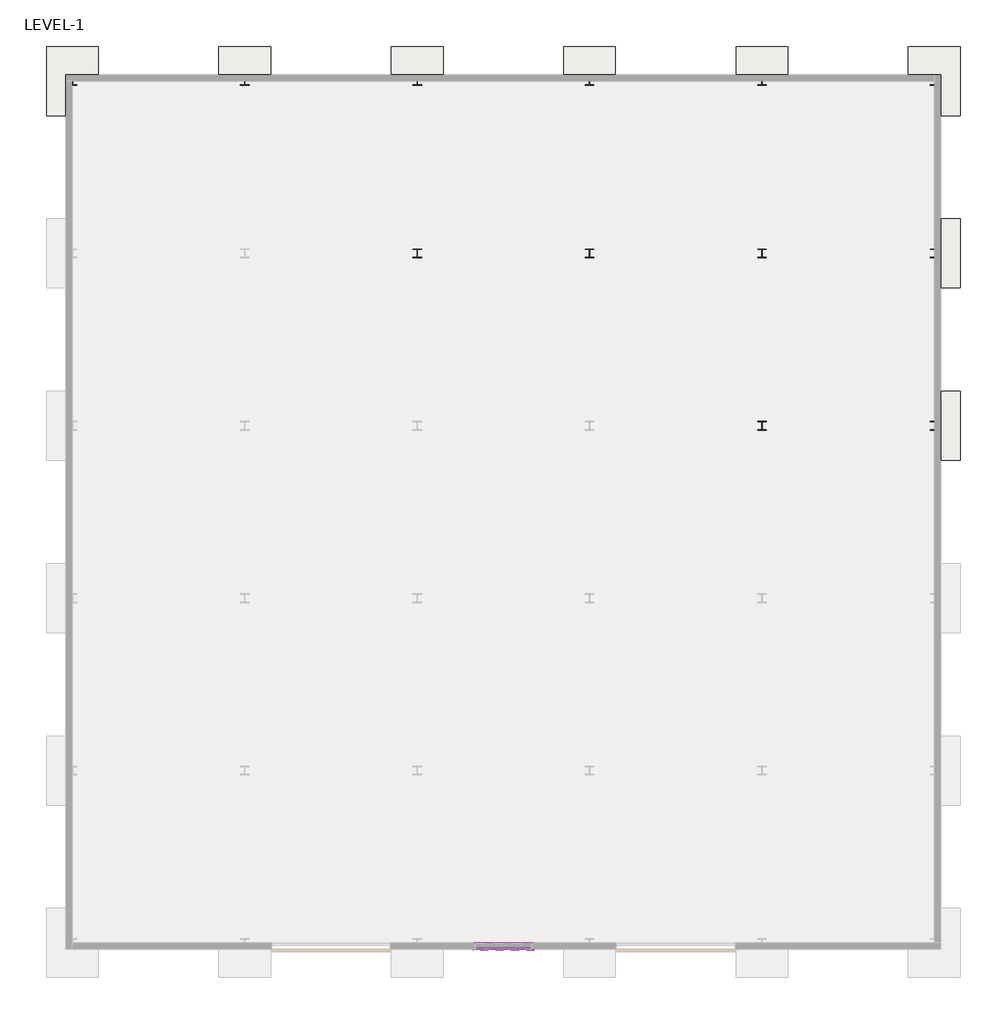
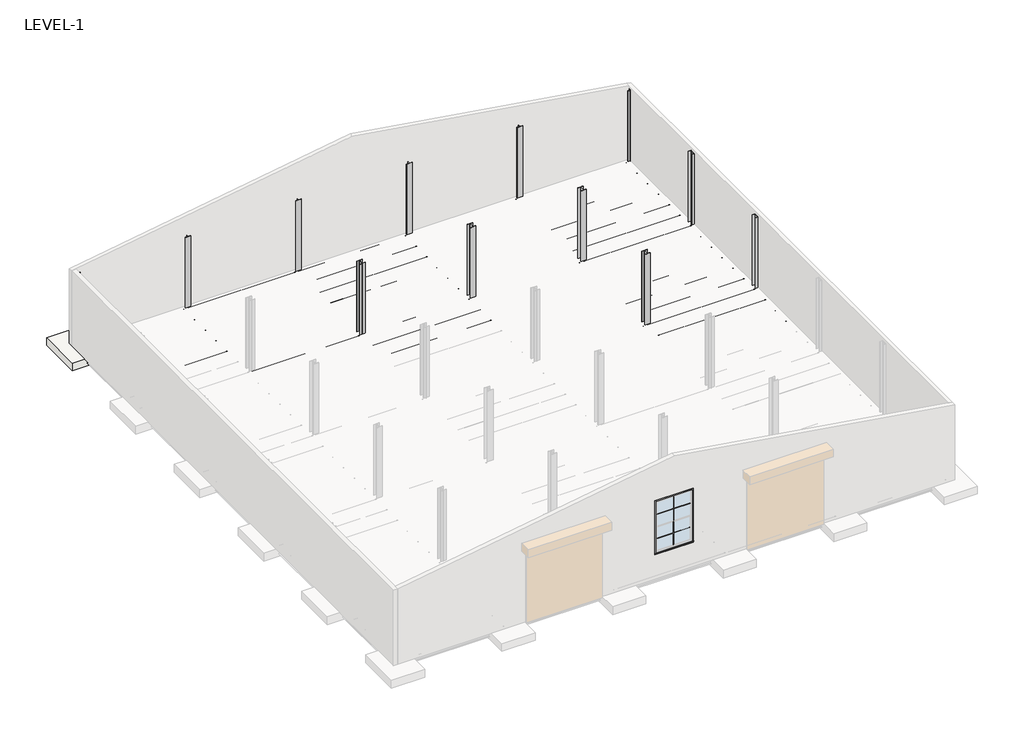
# One storey, part 3 of 3: 64 beams, 12 columns, 12 slabs, 4 proxies.
"""IFC4 building model written with IfcOpenShell, lengths in millimetres."""

from ifc_helpers import new_model, si_unit, origin, place, context, project, spatial, transform, mapped, element, save
from components import ub_universal_beams_ub305x165x40_15f88fa9, ub_universal_beams_ub305x165x40_f918ae41, ub_universal_beams_ub305x165x40_f15b2736, ub_universal_beams_ub305x165x40_44492b97, m_muntin_pattern_2x2_m_muntin_pattern_2x2_665a5da2, m_trim_window_exterior_flat_with_sill_5e8edc4f, m_trim_window_interior_flat_picture_frame_e5a503a4, uc_universal_columns_column_uc305x305x97_11a20181, slab_7b69f09a

model = new_model("IFC4")

# Units and contexts
model_context = context("Model", 3, world=origin())
ifc_project = project(units=[si_unit("LENGTHUNIT", "METRE", prefix="MILLI")], contexts=[model_context])

# Site, building, storey
site = spatial("IfcSite", under=ifc_project)
building = spatial("IfcBuilding", under=site)
storey = spatial("IfcBuildingStorey", under=building, Name="LEVEL-1", Elevation=0.0)

# Beams
placement = place(None, origin())
ub_universal_beams_ub305x165x40_shape = ub_universal_beams_ub305x165x40_15f88fa9(model_context)
element("IfcBeam", 1, ObjectType="UB-Universal Beams : UB305x165x40", at=placement, inside=storey, context=model_context, shape_type="MappedRepresentation", body=[
    mapped(ub_universal_beams_ub305x165x40_shape, transform((-15492.3332854, 15135.5234105, -151.7), x_axis=(1.0, 0.0, 0.0), y_axis=(0.0, 1.0, 0.0), z_axis=(0.0, 0.0, 1.0))),
])
element("IfcBeam", 2, ObjectType="UB-Universal Beams : UB305x165x40", at=placement, inside=storey, context=model_context, shape_type="MappedRepresentation", body=[
    mapped(ub_universal_beams_ub305x165x40_shape, transform((-15492.3332854, 14119.5234105, -151.7), x_axis=(1.0, 0.0, 0.0), y_axis=(0.0, 1.0, 0.0), z_axis=(0.0, 0.0, 1.0))),
])
element("IfcBeam", 3, ObjectType="UB-Universal Beams : UB305x165x40", at=placement, inside=storey, context=model_context, shape_type="MappedRepresentation", body=[
    mapped(ub_universal_beams_ub305x165x40_shape, transform((-15492.3332854, 13103.5234105, -151.7), x_axis=(1.0, 0.0, 0.0), y_axis=(0.0, 1.0, 0.0), z_axis=(0.0, 0.0, 1.0))),
])
element("IfcBeam", 4, ObjectType="UB-Universal Beams : UB305x165x40", at=placement, inside=storey, context=model_context, shape_type="MappedRepresentation", body=[
    mapped(ub_universal_beams_ub305x165x40_shape, transform((-15492.3332854, 12087.5234105, -151.7), x_axis=(1.0, 0.0, 0.0), y_axis=(0.0, 1.0, 0.0), z_axis=(0.0, 0.0, 1.0))),
])
element("IfcBeam", 5, ObjectType="UB-Universal Beams : UB305x165x40", at=placement, inside=storey, context=model_context, shape_type="MappedRepresentation", body=[
    mapped(ub_universal_beams_ub305x165x40_shape, transform((-3300.3332854, 15135.5234105, -151.7), x_axis=(1.0, 0.0, 0.0), y_axis=(0.0, 1.0, 0.0), z_axis=(0.0, 0.0, 1.0))),
])
element("IfcBeam", 6, ObjectType="UB-Universal Beams : UB305x165x40", at=placement, inside=storey, context=model_context, shape_type="MappedRepresentation", body=[
    mapped(ub_universal_beams_ub305x165x40_shape, transform((-3300.3332854, 14119.5234105, -151.7), x_axis=(1.0, 0.0, 0.0), y_axis=(0.0, 1.0, 0.0), z_axis=(0.0, 0.0, 1.0))),
])
element("IfcBeam", 7, ObjectType="UB-Universal Beams : UB305x165x40", at=placement, inside=storey, context=model_context, shape_type="MappedRepresentation", body=[
    mapped(ub_universal_beams_ub305x165x40_shape, transform((-3300.3332854, 13103.5234105, -151.7), x_axis=(1.0, 0.0, 0.0), y_axis=(0.0, 1.0, 0.0), z_axis=(0.0, 0.0, 1.0))),
])
element("IfcBeam", 8, ObjectType="UB-Universal Beams : UB305x165x40", at=placement, inside=storey, context=model_context, shape_type="MappedRepresentation", body=[
    mapped(ub_universal_beams_ub305x165x40_shape, transform((-3300.3332854, 12087.5234105, -151.7), x_axis=(1.0, 0.0, 0.0), y_axis=(0.0, 1.0, 0.0), z_axis=(0.0, 0.0, 1.0))),
])
element("IfcBeam", 9, ObjectType="UB-Universal Beams : UB305x165x40", at=placement, inside=storey, context=model_context, shape_type="MappedRepresentation", body=[
    mapped(ub_universal_beams_ub305x165x40_shape, transform((-3300.3332854, 11071.5234105, -151.7), x_axis=(1.0, 0.0, 0.0), y_axis=(0.0, 1.0, 0.0), z_axis=(0.0, 0.0, 1.0))),
])
element("IfcBeam", 10, ObjectType="UB-Universal Beams : UB305x165x40", at=placement, inside=storey, context=model_context, shape_type="MappedRepresentation", body=[
    mapped(ub_universal_beams_ub305x165x40_shape, transform((-3300.3332854, 9039.5234105, -151.7), x_axis=(1.0, 0.0, 0.0), y_axis=(0.0, 1.0, 0.0), z_axis=(0.0, 0.0, 1.0))),
])
element("IfcBeam", 11, ObjectType="UB-Universal Beams : UB305x165x40", at=placement, inside=storey, context=model_context, shape_type="MappedRepresentation", body=[
    mapped(ub_universal_beams_ub305x165x40_shape, transform((-3300.3332854, 8023.5234105, -151.7), x_axis=(1.0, 0.0, 0.0), y_axis=(0.0, 1.0, 0.0), z_axis=(0.0, 0.0, 1.0))),
])
element("IfcBeam", 12, ObjectType="UB-Universal Beams : UB305x165x40", at=placement, inside=storey, context=model_context, shape_type="MappedRepresentation", body=[
    mapped(ub_universal_beams_ub305x165x40_shape, transform((8891.6667146, 15135.5234105, -151.7), x_axis=(1.0, 0.0, 0.0), y_axis=(0.0, 1.0, 0.0), z_axis=(0.0, 0.0, 1.0))),
])
element("IfcBeam", 13, ObjectType="UB-Universal Beams : UB305x165x40", at=placement, inside=storey, context=model_context, shape_type="MappedRepresentation", body=[
    mapped(ub_universal_beams_ub305x165x40_shape, transform((8891.6667146, 14119.5234105, -151.7), x_axis=(1.0, 0.0, 0.0), y_axis=(0.0, 1.0, 0.0), z_axis=(0.0, 0.0, 1.0))),
])
element("IfcBeam", 14, ObjectType="UB-Universal Beams : UB305x165x40", at=placement, inside=storey, context=model_context, shape_type="MappedRepresentation", body=[
    mapped(ub_universal_beams_ub305x165x40_shape, transform((8891.6667146, 13103.5234105, -151.7), x_axis=(1.0, 0.0, 0.0), y_axis=(0.0, 1.0, 0.0), z_axis=(0.0, 0.0, 1.0))),
])
element("IfcBeam", 15, ObjectType="UB-Universal Beams : UB305x165x40", at=placement, inside=storey, context=model_context, shape_type="MappedRepresentation", body=[
    mapped(ub_universal_beams_ub305x165x40_shape, transform((8891.6667146, 12087.5234105, -151.7), x_axis=(1.0, 0.0, 0.0), y_axis=(0.0, 1.0, 0.0), z_axis=(0.0, 0.0, 1.0))),
])
element("IfcBeam", 16, ObjectType="UB-Universal Beams : UB305x165x40", at=placement, inside=storey, context=model_context, shape_type="MappedRepresentation", body=[
    mapped(ub_universal_beams_ub305x165x40_shape, transform((8891.6667146, 11071.5234105, -151.7), x_axis=(1.0, 0.0, 0.0), y_axis=(0.0, 1.0, 0.0), z_axis=(0.0, 0.0, 1.0))),
])
element("IfcBeam", 17, ObjectType="UB-Universal Beams : UB305x165x40", at=placement, inside=storey, context=model_context, shape_type="MappedRepresentation", body=[
    mapped(ub_universal_beams_ub305x165x40_shape, transform((8891.6667146, 9039.5234105, -151.7), x_axis=(1.0, 0.0, 0.0), y_axis=(0.0, 1.0, 0.0), z_axis=(0.0, 0.0, 1.0))),
])
element("IfcBeam", 18, ObjectType="UB-Universal Beams : UB305x165x40", at=placement, inside=storey, context=model_context, shape_type="MappedRepresentation", body=[
    mapped(ub_universal_beams_ub305x165x40_shape, transform((8891.6667146, 8023.5234105, -151.7), x_axis=(1.0, 0.0, 0.0), y_axis=(0.0, 1.0, 0.0), z_axis=(0.0, 0.0, 1.0))),
])
element("IfcBeam", 19, ObjectType="UB-Universal Beams : UB305x165x40", at=placement, inside=storey, context=model_context, shape_type="MappedRepresentation", body=[
    mapped(ub_universal_beams_ub305x165x40_shape, transform((8891.6667146, 7007.5234105, -151.7), x_axis=(1.0, 0.0, 0.0), y_axis=(0.0, 1.0, 0.0), z_axis=(0.0, 0.0, 1.0))),
])
element("IfcBeam", 20, ObjectType="UB-Universal Beams : UB305x165x40", at=placement, inside=storey, context=model_context, shape_type="MappedRepresentation", body=[
    mapped(ub_universal_beams_ub305x165x40_shape, transform((8891.6667146, 5991.5234105, -151.7), x_axis=(1.0, 0.0, 0.0), y_axis=(0.0, 1.0, 0.0), z_axis=(0.0, 0.0, 1.0))),
])
element("IfcBeam", 21, ObjectType="UB-Universal Beams : UB305x165x40", at=placement, inside=storey, context=model_context, shape_type="MappedRepresentation", body=[
    mapped(ub_universal_beams_ub305x165x40_shape, transform((8891.6667146, 4975.5234105, -151.7), x_axis=(1.0, 0.0, 0.0), y_axis=(0.0, 1.0, 0.0), z_axis=(0.0, 0.0, 1.0))),
])
element("IfcBeam", 22, ObjectType="UB-Universal Beams : UB305x165x40", at=placement, inside=storey, context=model_context, shape_type="MappedRepresentation", body=[
    mapped(ub_universal_beams_ub305x165x40_shape, transform((8891.6667146, 2943.5234105, -151.7), x_axis=(1.0, 0.0, 0.0), y_axis=(0.0, 1.0, 0.0), z_axis=(0.0, 0.0, 1.0))),
])
element("IfcBeam", 23, ObjectType="UB-Universal Beams : UB305x165x40", at=placement, inside=storey, context=model_context, shape_type="MappedRepresentation", body=[
    mapped(ub_universal_beams_ub305x165x40_shape, transform((8891.6667146, 1927.5234105, -151.7), x_axis=(1.0, 0.0, 0.0), y_axis=(0.0, 1.0, 0.0), z_axis=(0.0, 0.0, 1.0))),
])
element("IfcBeam", 24, ObjectType="UB-Universal Beams : UB305x165x40", at=placement, inside=storey, context=model_context, shape_type="MappedRepresentation", body=[
    mapped(ub_universal_beams_ub305x165x40_shape, transform((8891.6667146, 911.5234105, -151.7), x_axis=(1.0, 0.0, 0.0), y_axis=(0.0, 1.0, 0.0), z_axis=(0.0, 0.0, 1.0))),
])
element("IfcBeam", 25, ObjectType="UB-Universal Beams : UB305x165x40", at=placement, inside=storey, context=model_context, shape_type="MappedRepresentation", body=[
    mapped(ub_universal_beams_ub305x165x40_shape, transform((-7364.3332854, 13103.5234105, -151.7), x_axis=(0.0, -1.0, 0.0), y_axis=(1.0, 0.0, 0.0), z_axis=(0.0, 0.0, 1.0))),
])
element("IfcBeam", 26, ObjectType="UB-Universal Beams : UB305x165x40", at=placement, inside=storey, context=model_context, shape_type="MappedRepresentation", body=[
    mapped(ub_universal_beams_ub305x165x40_shape, transform((-8380.3332854, 13103.5234105, -151.7), x_axis=(0.0, -1.0, 0.0), y_axis=(1.0, 0.0, 0.0), z_axis=(0.0, 0.0, 1.0))),
])
element("IfcBeam", 27, ObjectType="UB-Universal Beams : UB305x165x40", at=placement, inside=storey, context=model_context, shape_type="MappedRepresentation", body=[
    mapped(ub_universal_beams_ub305x165x40_shape, transform((-9396.3332854, 13103.5234105, -151.7), x_axis=(0.0, -1.0, 0.0), y_axis=(1.0, 0.0, 0.0), z_axis=(0.0, 0.0, 1.0))),
])
element("IfcBeam", 28, ObjectType="UB-Universal Beams : UB305x165x40", at=placement, inside=storey, context=model_context, shape_type="MappedRepresentation", body=[
    mapped(ub_universal_beams_ub305x165x40_shape, transform((-10412.3332854, 13103.5234105, -151.7), x_axis=(0.0, -1.0, 0.0), y_axis=(1.0, 0.0, 0.0), z_axis=(0.0, 0.0, 1.0))),
])
element("IfcBeam", 29, ObjectType="UB-Universal Beams : UB305x165x40", at=placement, inside=storey, context=model_context, shape_type="MappedRepresentation", body=[
    mapped(ub_universal_beams_ub305x165x40_shape, transform((-11428.3332854, 13103.5234105, -151.7), x_axis=(0.0, -1.0, 0.0), y_axis=(1.0, 0.0, 0.0), z_axis=(0.0, 0.0, 1.0))),
])
element("IfcBeam", 30, ObjectType="UB-Universal Beams : UB305x165x40", at=placement, inside=storey, context=model_context, shape_type="MappedRepresentation", body=[
    mapped(ub_universal_beams_ub305x165x40_shape, transform((4827.6667146, 13103.5234105, -151.7), x_axis=(0.0, -1.0, 0.0), y_axis=(1.0, 0.0, 0.0), z_axis=(0.0, 0.0, 1.0))),
])
element("IfcBeam", 31, ObjectType="UB-Universal Beams : UB305x165x40", at=placement, inside=storey, context=model_context, shape_type="MappedRepresentation", body=[
    mapped(ub_universal_beams_ub305x165x40_shape, transform((3811.6667146, 13103.5234105, -151.7), x_axis=(0.0, -1.0, 0.0), y_axis=(1.0, 0.0, 0.0), z_axis=(0.0, 0.0, 1.0))),
])
element("IfcBeam", 32, ObjectType="UB-Universal Beams : UB305x165x40", at=placement, inside=storey, context=model_context, shape_type="MappedRepresentation", body=[
    mapped(ub_universal_beams_ub305x165x40_shape, transform((2795.6667146, 13103.5234105, -151.7), x_axis=(0.0, -1.0, 0.0), y_axis=(1.0, 0.0, 0.0), z_axis=(0.0, 0.0, 1.0))),
])
element("IfcBeam", 33, ObjectType="UB-Universal Beams : UB305x165x40", at=placement, inside=storey, context=model_context, shape_type="MappedRepresentation", body=[
    mapped(ub_universal_beams_ub305x165x40_shape, transform((1779.6667146, 13103.5234105, -151.7), x_axis=(0.0, -1.0, 0.0), y_axis=(1.0, 0.0, 0.0), z_axis=(0.0, 0.0, 1.0))),
])
element("IfcBeam", 34, ObjectType="UB-Universal Beams : UB305x165x40", at=placement, inside=storey, context=model_context, shape_type="MappedRepresentation", body=[
    mapped(ub_universal_beams_ub305x165x40_shape, transform((763.6667146, 13103.5234105, -151.7), x_axis=(0.0, -1.0, 0.0), y_axis=(1.0, 0.0, 0.0), z_axis=(0.0, 0.0, 1.0))),
])
element("IfcBeam", 35, ObjectType="UB-Universal Beams : UB305x165x40", at=placement, inside=storey, context=model_context, shape_type="MappedRepresentation", body=[
    mapped(ub_universal_beams_ub305x165x40_shape, transform((4827.6667146, 7007.5234105, -151.7), x_axis=(0.0, -1.0, 0.0), y_axis=(1.0, 0.0, 0.0), z_axis=(0.0, 0.0, 1.0))),
])
element("IfcBeam", 36, ObjectType="UB-Universal Beams : UB305x165x40", at=placement, inside=storey, context=model_context, shape_type="MappedRepresentation", body=[
    mapped(ub_universal_beams_ub305x165x40_shape, transform((3811.6667146, 7007.5234105, -151.7), x_axis=(0.0, -1.0, 0.0), y_axis=(1.0, 0.0, 0.0), z_axis=(0.0, 0.0, 1.0))),
])
element("IfcBeam", 37, ObjectType="UB-Universal Beams : UB305x165x40", at=placement, inside=storey, context=model_context, shape_type="MappedRepresentation", body=[
    mapped(ub_universal_beams_ub305x165x40_shape, transform((2795.6667146, 7007.5234105, -151.7), x_axis=(0.0, -1.0, 0.0), y_axis=(1.0, 0.0, 0.0), z_axis=(0.0, 0.0, 1.0))),
])
element("IfcBeam", 38, ObjectType="UB-Universal Beams : UB305x165x40", at=placement, inside=storey, context=model_context, shape_type="MappedRepresentation", body=[
    mapped(ub_universal_beams_ub305x165x40_shape, transform((1779.6667146, 7007.5234105, -151.7), x_axis=(0.0, -1.0, 0.0), y_axis=(1.0, 0.0, 0.0), z_axis=(0.0, 0.0, 1.0))),
])
element("IfcBeam", 39, ObjectType="UB-Universal Beams : UB305x165x40", at=placement, inside=storey, context=model_context, shape_type="MappedRepresentation", body=[
    mapped(ub_universal_beams_ub305x165x40_shape, transform((763.6667146, 7007.5234105, -151.7), x_axis=(0.0, -1.0, 0.0), y_axis=(1.0, 0.0, 0.0), z_axis=(0.0, 0.0, 1.0))),
])
element("IfcBeam", 40, ObjectType="UB-Universal Beams : UB305x165x40", at=placement, inside=storey, context=model_context, shape_type="MappedRepresentation", body=[
    mapped(ub_universal_beams_ub305x165x40_shape, transform((4827.6667146, 911.5234105, -151.7), x_axis=(0.0, -1.0, 0.0), y_axis=(1.0, 0.0, 0.0), z_axis=(0.0, 0.0, 1.0))),
])
element("IfcBeam", 41, ObjectType="UB-Universal Beams : UB305x165x40", at=placement, inside=storey, context=model_context, shape_type="MappedRepresentation", body=[
    mapped(ub_universal_beams_ub305x165x40_shape, transform((3811.6667146, 911.5234105, -151.7), x_axis=(0.0, -1.0, 0.0), y_axis=(1.0, 0.0, 0.0), z_axis=(0.0, 0.0, 1.0))),
])
element("IfcBeam", 42, ObjectType="UB-Universal Beams : UB305x165x40", at=placement, inside=storey, context=model_context, shape_type="MappedRepresentation", body=[
    mapped(ub_universal_beams_ub305x165x40_shape, transform((2795.6667146, 911.5234105, -151.7), x_axis=(0.0, -1.0, 0.0), y_axis=(1.0, 0.0, 0.0), z_axis=(0.0, 0.0, 1.0))),
])
element("IfcBeam", 43, ObjectType="UB-Universal Beams : UB305x165x40", at=placement, inside=storey, context=model_context, shape_type="MappedRepresentation", body=[
    mapped(ub_universal_beams_ub305x165x40_shape, transform((1779.6667146, 911.5234105, -151.7), x_axis=(0.0, -1.0, 0.0), y_axis=(1.0, 0.0, 0.0), z_axis=(0.0, 0.0, 1.0))),
])
element("IfcBeam", 44, ObjectType="UB-Universal Beams : UB305x165x40", at=placement, inside=storey, context=model_context, shape_type="MappedRepresentation", body=[
    mapped(ub_universal_beams_ub305x165x40_shape, transform((763.6667146, 911.5234105, -151.7), x_axis=(0.0, -1.0, 0.0), y_axis=(1.0, 0.0, 0.0), z_axis=(0.0, 0.0, 1.0))),
])
element("IfcBeam", 45, ObjectType="UB-Universal Beams : UB305x165x40", at=placement, inside=storey, context=model_context, shape_type="MappedRepresentation", body=[
    mapped(ub_universal_beams_ub305x165x40_shape, transform((2795.6667146, 3959.5234105, -151.7), x_axis=(1.0, 0.0, 0.0), y_axis=(0.0, 1.0, 0.0), z_axis=(0.0, 0.0, 1.0))),
])
element("IfcBeam", 46, ObjectType="UB-Universal Beams : UB305x165x40", at=placement, inside=storey, context=model_context, shape_type="MappedRepresentation", body=[
    mapped(ub_universal_beams_ub305x165x40_shape, transform((8891.6667146, 3959.5234105, -151.7), x_axis=(1.0, 0.0, 0.0), y_axis=(0.0, 1.0, 0.0), z_axis=(0.0, 0.0, 1.0))),
])
element("IfcBeam", 47, ObjectType="UB-Universal Beams : UB305x165x40", at=placement, inside=storey, context=model_context, shape_type="MappedRepresentation", body=[
    mapped(ub_universal_beams_ub305x165x40_shape, transform((-9396.3332854, 10055.5234105, -151.7), x_axis=(1.0, 0.0, 0.0), y_axis=(0.0, 1.0, 0.0), z_axis=(0.0, 0.0, 1.0))),
])
element("IfcBeam", 48, ObjectType="UB-Universal Beams : UB305x165x40", at=placement, inside=storey, context=model_context, shape_type="MappedRepresentation", body=[
    mapped(ub_universal_beams_ub305x165x40_shape, transform((-3300.3332854, 10055.5234105, -151.7), x_axis=(1.0, 0.0, 0.0), y_axis=(0.0, 1.0, 0.0), z_axis=(0.0, 0.0, 1.0))),
])
element("IfcBeam", 49, ObjectType="UB-Universal Beams : UB305x165x40", at=placement, inside=storey, context=model_context, shape_type="MappedRepresentation", body=[
    mapped(ub_universal_beams_ub305x165x40_shape, transform((2795.6667146, 10055.5234105, -151.7), x_axis=(1.0, 0.0, 0.0), y_axis=(0.0, 1.0, 0.0), z_axis=(0.0, 0.0, 1.0))),
])
element("IfcBeam", 50, ObjectType="UB-Universal Beams : UB305x165x40", at=placement, inside=storey, context=model_context, shape_type="MappedRepresentation", body=[
    mapped(ub_universal_beams_ub305x165x40_shape, transform((8891.6667146, 10055.5234105, -151.7), x_axis=(1.0, 0.0, 0.0), y_axis=(0.0, 1.0, 0.0), z_axis=(0.0, 0.0, 1.0))),
])
element("IfcBeam", 51, ObjectType="UB-Universal Beams : UB305x165x40", at=placement, inside=storey, context=model_context, shape_type="MappedRepresentation", body=[
    mapped(ub_universal_beams_ub305x165x40_shape, transform((-9396.3332854, 16151.5234105, -151.7), x_axis=(1.0, 0.0, 0.0), y_axis=(0.0, 1.0, 0.0), z_axis=(0.0, 0.0, 1.0))),
])
element("IfcBeam", 52, ObjectType="UB-Universal Beams : UB305x165x40", at=placement, inside=storey, context=model_context, shape_type="MappedRepresentation", body=[
    mapped(ub_universal_beams_ub305x165x40_shape, transform((-3300.3332854, 16151.5234105, -151.7), x_axis=(1.0, 0.0, 0.0), y_axis=(0.0, 1.0, 0.0), z_axis=(0.0, 0.0, 1.0))),
])
element("IfcBeam", 53, ObjectType="UB-Universal Beams : UB305x165x40", at=placement, inside=storey, context=model_context, shape_type="MappedRepresentation", body=[
    mapped(ub_universal_beams_ub305x165x40_shape, transform((2795.6667146, 16151.5234105, -151.7), x_axis=(1.0, 0.0, 0.0), y_axis=(0.0, 1.0, 0.0), z_axis=(0.0, 0.0, 1.0))),
])
element("IfcBeam", 54, ObjectType="UB-Universal Beams : UB305x165x40", at=placement, inside=storey, context=model_context, shape_type="MappedRepresentation", body=[
    mapped(ub_universal_beams_ub305x165x40_shape, transform((8891.6667146, 16151.5234105, -151.7), x_axis=(1.0, 0.0, 0.0), y_axis=(0.0, 1.0, 0.0), z_axis=(0.0, 0.0, 1.0))),
])
ub_universal_beams_ub305x165x40_2_shape = ub_universal_beams_ub305x165x40_f918ae41(model_context)
element("IfcBeam", 55, ObjectType="UB-Universal Beams : UB305x165x40", at=placement, inside=storey, context=model_context, shape_type="MappedRepresentation", body=[
    mapped(ub_universal_beams_ub305x165x40_2_shape, transform((11939.6667146, 911.5234105, -151.7), x_axis=(0.0, 1.0, 0.0), y_axis=(-1.0, 0.0, 0.0), z_axis=(0.0, 0.0, 1.0))),
])
element("IfcBeam", 56, ObjectType="UB-Universal Beams : UB305x165x40", at=placement, inside=storey, context=model_context, shape_type="MappedRepresentation", body=[
    mapped(ub_universal_beams_ub305x165x40_2_shape, transform((11939.6667146, 7007.5234105, -151.7), x_axis=(0.0, 1.0, 0.0), y_axis=(-1.0, 0.0, 0.0), z_axis=(0.0, 0.0, 1.0))),
])
element("IfcBeam", 57, ObjectType="UB-Universal Beams : UB305x165x40", at=placement, inside=storey, context=model_context, shape_type="MappedRepresentation", body=[
    mapped(ub_universal_beams_ub305x165x40_2_shape, transform((5843.6667146, 911.5234105, -151.7), x_axis=(0.0, 1.0, 0.0), y_axis=(-1.0, 0.0, 0.0), z_axis=(0.0, 0.0, 1.0))),
])
element("IfcBeam", 58, ObjectType="UB-Universal Beams : UB305x165x40", at=placement, inside=storey, context=model_context, shape_type="MappedRepresentation", body=[
    mapped(ub_universal_beams_ub305x165x40_2_shape, transform((5843.6667146, 7007.5234105, -151.7), x_axis=(0.0, 1.0, 0.0), y_axis=(-1.0, 0.0, 0.0), z_axis=(0.0, 0.0, 1.0))),
])
ub_universal_beams_ub305x165x40_3_shape = ub_universal_beams_ub305x165x40_f15b2736(model_context)
element("IfcBeam", 59, ObjectType="UB-Universal Beams : UB305x165x40", at=placement, inside=storey, context=model_context, shape_type="MappedRepresentation", body=[
    mapped(ub_universal_beams_ub305x165x40_3_shape, transform((-15549.3308854, 16151.5234105, -151.7), x_axis=(1.0, 0.0, 0.0), y_axis=(0.0, 1.0, 0.0), z_axis=(0.0, 0.0, 1.0))),
])
ub_universal_beams_ub305x165x40_4_shape = ub_universal_beams_ub305x165x40_44492b97(model_context)
element("IfcBeam", 60, ObjectType="UB-Universal Beams : UB305x165x40", at=placement, inside=storey, context=model_context, shape_type="MappedRepresentation", body=[
    mapped(ub_universal_beams_ub305x165x40_4_shape, transform((11939.6667146, 13160.6734105, -151.7), x_axis=(0.0, 1.0, 0.0), y_axis=(-1.0, 0.0, 0.0), z_axis=(0.0, 0.0, 1.0))),
])
element("IfcBeam", 61, ObjectType="UB-Universal Beams : UB305x165x40", at=placement, inside=storey, context=model_context, shape_type="MappedRepresentation", body=[
    mapped(ub_universal_beams_ub305x165x40_4_shape, transform((5843.6667146, 13160.6734105, -151.7), x_axis=(0.0, 1.0, 0.0), y_axis=(-1.0, 0.0, 0.0), z_axis=(0.0, 0.0, 1.0))),
])
element("IfcBeam", 62, ObjectType="UB-Universal Beams : UB305x165x40", at=placement, inside=storey, context=model_context, shape_type="MappedRepresentation", body=[
    mapped(ub_universal_beams_ub305x165x40_4_shape, transform((-252.3332854, 13160.6734105, -151.7), x_axis=(0.0, 1.0, 0.0), y_axis=(-1.0, 0.0, 0.0), z_axis=(0.0, 0.0, 1.0))),
])
element("IfcBeam", 63, ObjectType="UB-Universal Beams : UB305x165x40", at=placement, inside=storey, context=model_context, shape_type="MappedRepresentation", body=[
    mapped(ub_universal_beams_ub305x165x40_4_shape, transform((-6348.3332854, 13160.6734105, -151.7), x_axis=(0.0, 1.0, 0.0), y_axis=(-1.0, 0.0, 0.0), z_axis=(0.0, 0.0, 1.0))),
])
element("IfcBeam", 64, ObjectType="UB-Universal Beams : UB305x165x40", at=placement, inside=storey, context=model_context, shape_type="MappedRepresentation", body=[
    mapped(ub_universal_beams_ub305x165x40_4_shape, transform((-12444.3332854, 13160.6734105, -151.7), x_axis=(0.0, 1.0, 0.0), y_axis=(-1.0, 0.0, 0.0), z_axis=(0.0, 0.0, 1.0))),
])

# Proxies
m_muntin_pattern_2x2_m_muntin_pattern_2x2_shape = m_muntin_pattern_2x2_m_muntin_pattern_2x2_665a5da2(model_context)
element("IfcBuildingElementProxy", 65, Name="M_Muntin Pattern_2x2 : M_Muntin Pattern_2x2", ObjectType="M_Muntin Pattern_2x2 : M_Muntin Pattern_2x2", at=placement, inside=storey, context=model_context, shape_type="MappedRepresentation", body=[
    mapped(m_muntin_pattern_2x2_m_muntin_pattern_2x2_shape, transform((-3300.3332854, -14522.1515895, 3035.1090152), x_axis=(-1.0, 0.0, 0.0), y_axis=(0.0, -1.0, 0.0), z_axis=(0.0, 0.0, 1.0))),
])
element("IfcBuildingElementProxy", 66, Name="M_Muntin Pattern_2x2 : M_Muntin Pattern_2x2", ObjectType="M_Muntin Pattern_2x2 : M_Muntin Pattern_2x2", at=placement, inside=storey, context=model_context, shape_type="MappedRepresentation", body=[
    mapped(m_muntin_pattern_2x2_m_muntin_pattern_2x2_shape, transform((-3300.3332854, -14477.7015895, 1589.0840152), x_axis=(-1.0, 0.0, 0.0), y_axis=(0.0, -1.0, 0.0), z_axis=(0.0, 0.0, 1.0))),
])
m_trim_window_exterior_flat_with_sill_shape = m_trim_window_exterior_flat_with_sill_5e8edc4f(model_context)
element("IfcBuildingElementProxy", 67, Name="M_Trim-Window-Exterior-Flat : with Sill", ObjectType="M_Trim-Window-Exterior-Flat : with Sill", at=placement, inside=storey, context=model_context, shape_type="MappedRepresentation", body=[
    mapped(m_trim_window_exterior_flat_with_sill_shape, transform((-3300.3332854, -14557.0765895, 4512.8840152), x_axis=(1.0, 0.0, 0.0), y_axis=(0.0, 0.0, 1.0), z_axis=(0.0, -1.0, 0.0))),
])
m_trim_window_interior_flat_picture_frame_shape = m_trim_window_interior_flat_picture_frame_e5a503a4(model_context)
element("IfcBuildingElementProxy", 68, Name="M_Trim-Window-Interior-Flat : Picture Frame", ObjectType="M_Trim-Window-Interior-Flat : Picture Frame", at=placement, inside=storey, context=model_context, shape_type="MappedRepresentation", body=[
    mapped(m_trim_window_interior_flat_picture_frame_shape, transform((-3300.3332854, -14328.4765895, 4512.8840152), x_axis=(-1.0, 0.0, 0.0), y_axis=(0.0, 0.0, 1.0), z_axis=(0.0, 1.0, 0.0))),
])

# Columns
uc_universal_columns_column_uc305x305x97_shape = uc_universal_columns_column_uc305x305x97_11a20181(model_context)
element("IfcColumn", 69, ObjectType="UC-Universal Columns-Column : UC305x305x97", at=placement, inside=storey, context=model_context, shape_type="MappedRepresentation", body=[
    mapped(uc_universal_columns_column_uc305x305x97_shape, transform((11939.6667146, 3959.5234105, 0.0), x_axis=(1.0, 0.0, 0.0), y_axis=(0.0, 1.0, 0.0), z_axis=(0.0, 0.0, 1.0))),
])
element("IfcColumn", 70, ObjectType="UC-Universal Columns-Column : UC305x305x97", at=placement, inside=storey, context=model_context, shape_type="MappedRepresentation", body=[
    mapped(uc_universal_columns_column_uc305x305x97_shape, transform((5843.6667146, 3959.5234105, 0.0), x_axis=(1.0, 0.0, 0.0), y_axis=(0.0, 1.0, 0.0), z_axis=(0.0, 0.0, 1.0))),
])
element("IfcColumn", 71, ObjectType="UC-Universal Columns-Column : UC305x305x97", at=placement, inside=storey, context=model_context, shape_type="MappedRepresentation", body=[
    mapped(uc_universal_columns_column_uc305x305x97_shape, transform((11939.6667146, 10055.5234105, 0.0), x_axis=(1.0, 0.0, 0.0), y_axis=(0.0, 1.0, 0.0), z_axis=(0.0, 0.0, 1.0))),
])
element("IfcColumn", 72, ObjectType="UC-Universal Columns-Column : UC305x305x97", at=placement, inside=storey, context=model_context, shape_type="MappedRepresentation", body=[
    mapped(uc_universal_columns_column_uc305x305x97_shape, transform((5843.6667146, 10055.5234105, 0.0), x_axis=(1.0, 0.0, 0.0), y_axis=(0.0, 1.0, 0.0), z_axis=(0.0, 0.0, 1.0))),
])
element("IfcColumn", 73, ObjectType="UC-Universal Columns-Column : UC305x305x97", at=placement, inside=storey, context=model_context, shape_type="MappedRepresentation", body=[
    mapped(uc_universal_columns_column_uc305x305x97_shape, transform((-252.3332854, 10055.5234105, 0.0), x_axis=(1.0, 0.0, 0.0), y_axis=(0.0, 1.0, 0.0), z_axis=(0.0, 0.0, 1.0))),
])
element("IfcColumn", 74, ObjectType="UC-Universal Columns-Column : UC305x305x97", at=placement, inside=storey, context=model_context, shape_type="MappedRepresentation", body=[
    mapped(uc_universal_columns_column_uc305x305x97_shape, transform((-6348.3332854, 10055.5234105, 0.0), x_axis=(1.0, 0.0, 0.0), y_axis=(0.0, 1.0, 0.0), z_axis=(0.0, 0.0, 1.0))),
])
element("IfcColumn", 75, ObjectType="UC-Universal Columns-Column : UC305x305x97", at=placement, inside=storey, context=model_context, shape_type="MappedRepresentation", body=[
    mapped(uc_universal_columns_column_uc305x305x97_shape, transform((11939.6667146, 16151.5234105, 0.0), x_axis=(1.0, 0.0, 0.0), y_axis=(0.0, 1.0, 0.0), z_axis=(0.0, 0.0, 1.0))),
])
element("IfcColumn", 76, ObjectType="UC-Universal Columns-Column : UC305x305x97", at=placement, inside=storey, context=model_context, shape_type="MappedRepresentation", body=[
    mapped(uc_universal_columns_column_uc305x305x97_shape, transform((5843.6667146, 16151.5234105, 0.0), x_axis=(1.0, 0.0, 0.0), y_axis=(0.0, 1.0, 0.0), z_axis=(0.0, 0.0, 1.0))),
])
element("IfcColumn", 77, ObjectType="UC-Universal Columns-Column : UC305x305x97", at=placement, inside=storey, context=model_context, shape_type="MappedRepresentation", body=[
    mapped(uc_universal_columns_column_uc305x305x97_shape, transform((-252.3332854, 16151.5234105, 0.0), x_axis=(1.0, 0.0, 0.0), y_axis=(0.0, 1.0, 0.0), z_axis=(0.0, 0.0, 1.0))),
])
element("IfcColumn", 78, ObjectType="UC-Universal Columns-Column : UC305x305x97", at=placement, inside=storey, context=model_context, shape_type="MappedRepresentation", body=[
    mapped(uc_universal_columns_column_uc305x305x97_shape, transform((-6348.3332854, 16151.5234105, 0.0), x_axis=(1.0, 0.0, 0.0), y_axis=(0.0, 1.0, 0.0), z_axis=(0.0, 0.0, 1.0))),
])
element("IfcColumn", 79, ObjectType="UC-Universal Columns-Column : UC305x305x97", at=placement, inside=storey, context=model_context, shape_type="MappedRepresentation", body=[
    mapped(uc_universal_columns_column_uc305x305x97_shape, transform((-12444.3332854, 16151.5234105, 0.0), x_axis=(1.0, 0.0, 0.0), y_axis=(0.0, 1.0, 0.0), z_axis=(0.0, 0.0, 1.0))),
])
element("IfcColumn", 80, ObjectType="UC-Universal Columns-Column : UC305x305x97", at=placement, inside=storey, context=model_context, shape_type="MappedRepresentation", body=[
    mapped(uc_universal_columns_column_uc305x305x97_shape, transform((-18540.3332854, 16151.5234105, 0.0), x_axis=(1.0, 0.0, 0.0), y_axis=(0.0, 1.0, 0.0), z_axis=(0.0, 0.0, 1.0))),
])

# Slabs
slab_shape = slab_7b69f09a(model_context)
element("IfcSlab", 81, ObjectType="Footing-Rectangular : 96\" x 72\" x 18\"", at=placement, inside=storey, context=model_context, shape_type="MappedRepresentation", body=[
    mapped(slab_shape, transform((11939.6667146, 3959.5234105, 0.0), x_axis=(1.0, 0.0, 0.0), y_axis=(0.0, 1.0, 0.0), z_axis=(0.0, 0.0, 1.0))),
])
element("IfcSlab", 82, ObjectType="Footing-Rectangular : 96\" x 72\" x 18\"", at=placement, inside=storey, context=model_context, shape_type="MappedRepresentation", body=[
    mapped(slab_shape, transform((5843.6667146, 3959.5234105, 0.0), x_axis=(1.0, 0.0, 0.0), y_axis=(0.0, 1.0, 0.0), z_axis=(0.0, 0.0, 1.0))),
])
element("IfcSlab", 83, ObjectType="Footing-Rectangular : 96\" x 72\" x 18\"", at=placement, inside=storey, context=model_context, shape_type="MappedRepresentation", body=[
    mapped(slab_shape, transform((11939.6667146, 10055.5234105, 0.0), x_axis=(1.0, 0.0, 0.0), y_axis=(0.0, 1.0, 0.0), z_axis=(0.0, 0.0, 1.0))),
])
element("IfcSlab", 84, ObjectType="Footing-Rectangular : 96\" x 72\" x 18\"", at=placement, inside=storey, context=model_context, shape_type="MappedRepresentation", body=[
    mapped(slab_shape, transform((5843.6667146, 10055.5234105, 0.0), x_axis=(1.0, 0.0, 0.0), y_axis=(0.0, 1.0, 0.0), z_axis=(0.0, 0.0, 1.0))),
])
element("IfcSlab", 85, ObjectType="Footing-Rectangular : 96\" x 72\" x 18\"", at=placement, inside=storey, context=model_context, shape_type="MappedRepresentation", body=[
    mapped(slab_shape, transform((-252.3332854, 10055.5234105, 0.0), x_axis=(1.0, 0.0, 0.0), y_axis=(0.0, 1.0, 0.0), z_axis=(0.0, 0.0, 1.0))),
])
element("IfcSlab", 86, ObjectType="Footing-Rectangular : 96\" x 72\" x 18\"", at=placement, inside=storey, context=model_context, shape_type="MappedRepresentation", body=[
    mapped(slab_shape, transform((-6348.3332854, 10055.5234105, 0.0), x_axis=(1.0, 0.0, 0.0), y_axis=(0.0, 1.0, 0.0), z_axis=(0.0, 0.0, 1.0))),
])
element("IfcSlab", 87, ObjectType="Footing-Rectangular : 96\" x 72\" x 18\"", at=placement, inside=storey, context=model_context, shape_type="MappedRepresentation", body=[
    mapped(slab_shape, transform((11939.6667146, 16151.5234105, 0.0), x_axis=(1.0, 0.0, 0.0), y_axis=(0.0, 1.0, 0.0), z_axis=(0.0, 0.0, 1.0))),
])
element("IfcSlab", 88, ObjectType="Footing-Rectangular : 96\" x 72\" x 18\"", at=placement, inside=storey, context=model_context, shape_type="MappedRepresentation", body=[
    mapped(slab_shape, transform((5843.6667146, 16151.5234105, 0.0), x_axis=(1.0, 0.0, 0.0), y_axis=(0.0, 1.0, 0.0), z_axis=(0.0, 0.0, 1.0))),
])
element("IfcSlab", 89, ObjectType="Footing-Rectangular : 96\" x 72\" x 18\"", at=placement, inside=storey, context=model_context, shape_type="MappedRepresentation", body=[
    mapped(slab_shape, transform((-252.3332854, 16151.5234105, 0.0), x_axis=(1.0, 0.0, 0.0), y_axis=(0.0, 1.0, 0.0), z_axis=(0.0, 0.0, 1.0))),
])
element("IfcSlab", 90, ObjectType="Footing-Rectangular : 96\" x 72\" x 18\"", at=placement, inside=storey, context=model_context, shape_type="MappedRepresentation", body=[
    mapped(slab_shape, transform((-6348.3332854, 16151.5234105, 0.0), x_axis=(1.0, 0.0, 0.0), y_axis=(0.0, 1.0, 0.0), z_axis=(0.0, 0.0, 1.0))),
])
element("IfcSlab", 91, ObjectType="Footing-Rectangular : 96\" x 72\" x 18\"", at=placement, inside=storey, context=model_context, shape_type="MappedRepresentation", body=[
    mapped(slab_shape, transform((-12444.3332854, 16151.5234105, 0.0), x_axis=(1.0, 0.0, 0.0), y_axis=(0.0, 1.0, 0.0), z_axis=(0.0, 0.0, 1.0))),
])
element("IfcSlab", 92, ObjectType="Footing-Rectangular : 96\" x 72\" x 18\"", at=placement, inside=storey, context=model_context, shape_type="MappedRepresentation", body=[
    mapped(slab_shape, transform((-18540.3332854, 16151.5234105, 0.0), x_axis=(1.0, 0.0, 0.0), y_axis=(0.0, 1.0, 0.0), z_axis=(0.0, 0.0, 1.0))),
])

save(model, "model.ifc")

# Revit data of these elements
# Type "UB-Universal Beams : UB305x165x40"
#   Section Name Key = "UB305X165X40"
#   Width = 16.5 cm
#   Web Thickness = 0.6 cm
#   Web Fillet = 0.89 cm
#   Warping Constant = 164000.0 cm⁶
#   Torsional Moment of Inertia = 14.70 cm⁴
#   Section Area = 51.3 cm²
#   Plastic Modulus weak axis = 142.0 cm³
#   Plastic Modulus strong axis = 623.0 cm³
#   Nominal Weight = 40.2999 kgf/m
#   Moment of Inertia weak axis = 764.00 cm⁴
#   Moment of Inertia strong axis = 8503.00 cm⁴
#   Height = 30.34 cm
#   Flange Thickness = 1.02 cm
#   Elastic Modulus weak axis = 92.6 cm³
#   Elastic Modulus strong axis = 560.0 cm³
#   Centroid Vertical = 15.17 cm
#   Centroid Horizontal = 8.25 cm
#   Bolt Spacing = 9.0 cm
#   Length [instance default] = 1500 mm
#   Structural Material [instance default] = Metal - Steel 43-275
#   Type Comments = ""
#   Assembly Code = ""
# Type "M_Muntin Pattern_2x2 : M_Muntin Pattern_2x2"
#   Width [instance default] = 1200 mm
#   Thickness = 12.7 mm
#   Height [instance default] = 1200 mm
#   Distance = 19.05 mm
#   Interior Material [instance default] = none
#   Exterior Material [instance default] = none
#   Default Elevation = 0
# Type "M_Trim-Window-Exterior-Flat : with Sill"
#   Trim Width = 60 mm
#   Trim Thickness_Picture Frame = 30 mm
#   Trim Thickness_with Sill = 19.05 mm
#   Sill Thickness = 30 mm
#   Opening Width [instance default] = 600 mm
#   Opening Height [instance default] = 900 mm
#   Default Elevation = 1200 mm
#   Sill = yes
#   Picture Frame = no
#   Trim Material [instance default] = none
# Type "M_Trim-Window-Interior-Flat : Picture Frame"
#   Trim Thickness_Picture Frame = 30 mm
#   Trim Width = 60 mm
#   Trim Thickness_with Sill = 20 mm
#   Sill Thickness = 30 mm
#   Opening Width [instance default] = 600 mm
#   Opening Height [instance default] = 900 mm
#   Default Elevation = 1200 mm
#   Sill = no
#   Picture Frame = yes
#   Trim Material [instance default] = none
# Type "UC-Universal Columns-Column : UC305x305x97"
#   Section Name Key = "UC305x305x97"
#   Width = 30.53 cm
#   Web Thickness = 0.99 cm
#   Web Fillet = 1.52 cm
#   Warping Constant = 1560000.0 cm⁶
#   Torsional Moment of Inertia = 91.20 cm⁴
#   Section Area = 123.0 cm²
#   Plastic Modulus weak axis = 726.0 cm³
#   Plastic Modulus strong axis = 1592.0 cm³
#   Nominal Weight = 96.8996 kgf/m
#   Moment of Inertia weak axis = 7308.00 cm⁴
#   Moment of Inertia strong axis = 22249.00 cm⁴
#   Height = 30.79 cm
#   Flange Thickness = 1.54 cm
#   Elastic Modulus weak axis = 479.0 cm³
#   Elastic Modulus strong axis = 1445.0 cm³
#   Centroid Vertical = 15.395 cm
#   Centroid Horizontal = 15.265 cm
#   Bolt Spacing = 14.0 cm
#   Structural Material [instance default] = Metal - Steel 43-275
#   Type Comments = ""
#   Assembly Code = ""
# Type "Footing-Rectangular : 96\" x 72\" x 18\""
#   Assembly Code = "A1010100"
#   Width = 1828.8 mm
#   Length = 2438.4 mm
#   Foundation Thickness = 457.2 mm
#   Structural Material [instance default] = Concrete, Cast-in-Place gray
# Elements 1, 2, 3, 4, 5, 6, 7, 8, 9, 10, 11, 12, 13, 14, 15, 16, 17, 18, 19, 20, 21, 22, 23, 24, 25, 26, 27, 28, 29, 30, 31, 32, 33, 34, 35, 36, 37, 38, 39, 40, 41, 42, 43, 44, 45, 46, 47, 48, 49, 50, 51, 52, 53, 54, 55, 56, 57, 58, 59, 60, 61, 62, 63, 64 (IfcBeam, "UB-Universal Beams : UB305x165x40")
#   Structural Material = Metal - Steel 43-275
#   Phase Created = New Construction
#   Materials on its faces: "Metal - Steel 43-275"
# Elements 65, 66 (IfcBuildingElementProxy, "M_Muntin Pattern_2x2 : M_Muntin Pattern_2x2")
#   Width = 1847.6 mm
#   Height = 1401.575 mm
#   Interior Material = Wood - Stained
#   Exterior Material = Clad - White
#   Phase Created = New Construction
#   Materials on its faces: "Clad - White", "Wood - Stained"
# Element 67 (IfcBuildingElementProxy, "M_Trim-Window-Exterior-Flat : with Sill")
#   Opening Width = 2000 mm
#   Opening Height = 3000 mm
#   Trim Material = Clad - White
#   Phase Created = New Construction
#   Materials on its faces: "Clad - White"
# Element 68 (IfcBuildingElementProxy, "M_Trim-Window-Interior-Flat : Picture Frame")
#   Opening Width = 2000 mm
#   Opening Height = 3000 mm
#   Trim Material = Wood - Stained
#   Phase Created = New Construction
#   Materials on its faces: "Wood - Stained"
# Elements 69, 70, 71, 72, 73, 74, 75, 76, 77, 78, 79, 80 (IfcColumn, "UC-Universal Columns-Column : UC305x305x97")
#   Structural Material = Metal - Steel 43-275
#   Phase Created = New Construction
#   Materials on its faces: "Metal - Steel 43-275"
# Elements 81, 82, 83, 84, 85, 86, 87, 88, 89, 90, 91, 92 (IfcSlab, "Footing-Rectangular : 96\" x 72\" x 18\"")
#   Structural Material = Concrete, Cast-in-Place gray
#   Phase Created = New Construction
#   Materials on its faces: "Concrete, Cast-in-Place gray"
# Materials
#   "Metal - Steel 43-275": class "Metal", colour RGB 247 247 247, transparency 0, Cost = 0
#   "Concrete, Cast-in-Place gray": class "Concrete", colour RGB 192 192 192, transparency 0, Description = "Cast-in-place concrete", Cost = 0
#   "Clad - White": class "Wood", colour RGB 242 242 238, transparency 0, Cost = 0
#   "Wood - Stained": class "Wood", colour RGB 224 178 126, transparency 0, Cost = 0
